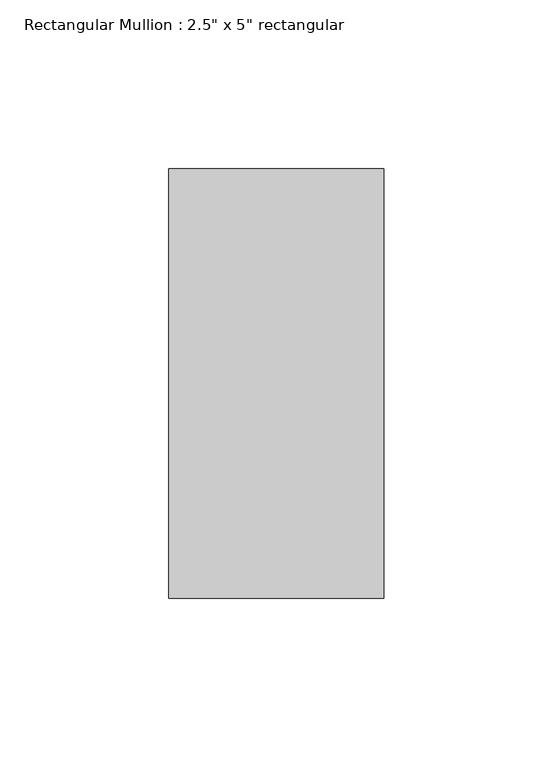
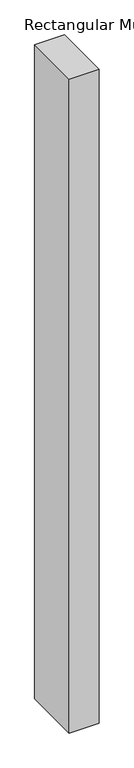
"""IFC4 building model written with IfcOpenShell, lengths in millimetres: member geometry."""

from ifc_helpers import new_model, si_unit, frame, origin, place, context, project, spatial, polyline, outline, extrude, source, transform, mapped, element, save


def member_91d29dfe(model_context):
    return source(origin(), model_context, "Body", "SweptSolid", [
        extrude(outline(polyline([(0.0, 63.5), (0.0, -63.5), (-63.5, -63.5), (-63.5, 63.5), (0.0, 63.5)])), frame((0.0, 0.0, -1468.7815981), z_axis=(0.0, 0.0, 1.0), x_axis=(1.0, 0.0, 0.0)), (0.0, 0.0, 1.0), 1468.7815981),
    ])


if __name__ == "__main__":
    model = new_model("IFC4")
    model_context = context("Model", 3, world=origin())
    ifc_project = project(units=[si_unit("LENGTHUNIT", "METRE", prefix="MILLI")], contexts=[model_context])
    site = spatial("IfcSite", under=ifc_project)
    building = spatial("IfcBuilding", under=site)
    placement = place(None, origin())
    member_shape = member_91d29dfe(model_context)
    element("IfcMember", 1, ObjectType="Rectangular Mullion : 2.5\" x 5\" rectangular", at=placement, inside=building, context=model_context, shape_type="MappedRepresentation", body=[
        mapped(member_shape, transform((0.0, 0.0, 0.0), x_axis=(1.0, 0.0, 0.0), y_axis=(0.0, 1.0, 0.0), z_axis=(0.0, 0.0, 1.0))),
    ])
    save(model, "model.ifc")

# Revit data of these elements
# Type "Rectangular Mullion : 2.5\" x 5\" rectangular"
#   built-in parameter 1007304 = 0.416667 (stored number, unit not read)
#   built-in parameter 1007301 = 0.104167 (stored number, unit not read)
#   built-in parameter 1007300 = 0.104167 (stored number, unit not read)
# Element 1 (IfcMember, "Rectangular Mullion : 2.5\" x 5\" rectangular")
#   Materials on its faces: "Aluminum"
# Materials
#   "Aluminum": class "Metal", colour RGB 247 247 247, transparency 0, Description = "Aluminum 6061", Cost = 0
